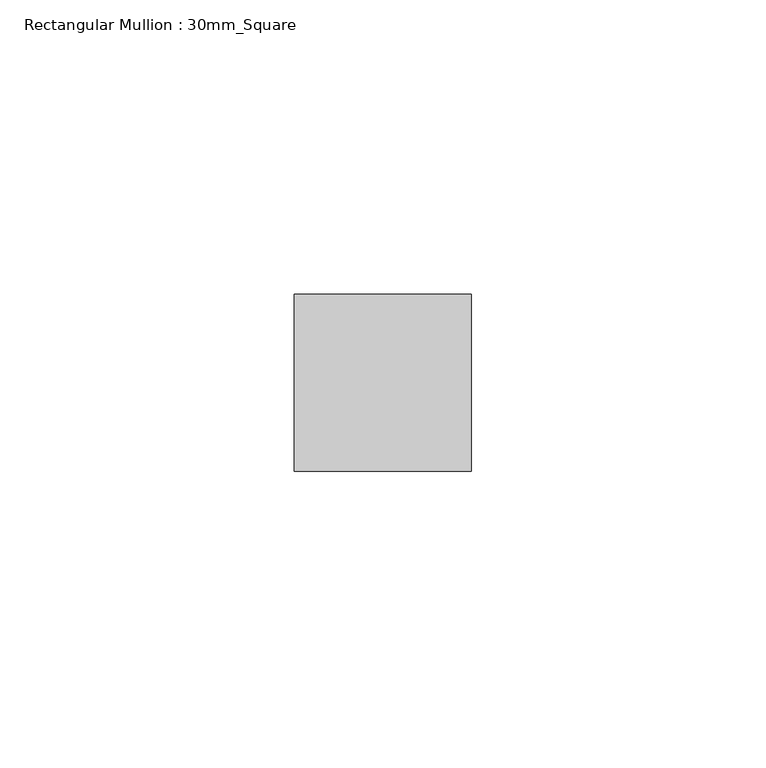
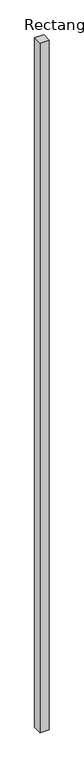
"""IFC4 building model written with IfcOpenShell, lengths in millimetres: member geometry, Rectangular Mullion : 30mm_Square."""

from ifc_helpers import new_model, si_unit, frame, origin, place, context, project, spatial, polyline, outline, extrude, source, transform, mapped, element, save


def rectangular_mullion_30mm_square_6919c9ce(model_context):
    return source(origin(), model_context, "Body", "SweptSolid", [
        extrude(outline(polyline([(0.0, 15.0), (0.0, -15.0), (-30.0, -15.0), (-30.0, 15.0), (0.0, 15.0)])), frame((0.0, 0.0, -2400.0242188), z_axis=(0.0, 0.0, 1.0), x_axis=(1.0, 0.0, 0.0)), (0.0, 0.0, 1.0), 2400.0242188),
    ])


if __name__ == "__main__":
    model = new_model("IFC4")
    model_context = context("Model", 3, world=origin())
    ifc_project = project(units=[si_unit("LENGTHUNIT", "METRE", prefix="MILLI")], contexts=[model_context])
    site = spatial("IfcSite", under=ifc_project)
    building = spatial("IfcBuilding", under=site)
    placement = place(None, origin())
    rectangular_mullion_30mm_square_shape = rectangular_mullion_30mm_square_6919c9ce(model_context)
    element("IfcMember", 1, ObjectType="Rectangular Mullion : 30mm_Square", at=placement, inside=building, context=model_context, shape_type="MappedRepresentation", body=[
        mapped(rectangular_mullion_30mm_square_shape, transform((0.0, 0.0, 0.0), x_axis=(1.0, 0.0, 0.0), y_axis=(0.0, 1.0, 0.0), z_axis=(0.0, 0.0, 1.0))),
    ])
    save(model, "model.ifc")

# Revit data of these elements
# Type "Rectangular Mullion : 30mm_Square"
#   Keynote = "H11"
#   built-in parameter 1007304 = 0.0984252 (stored number, unit not read)
#   built-in parameter 1007301 = 0.0492126 (stored number, unit not read)
#   built-in parameter 1007300 = 0.0492126 (stored number, unit not read)
# Element 1 (IfcMember, "Rectangular Mullion : 30mm_Square")
#   Materials on its faces: "Aluminium"
# Materials
#   "Aluminium": class "Metal", colour RGB 247 247 247, transparency 0, Description = "Aluminium 6061", Cost = 0
